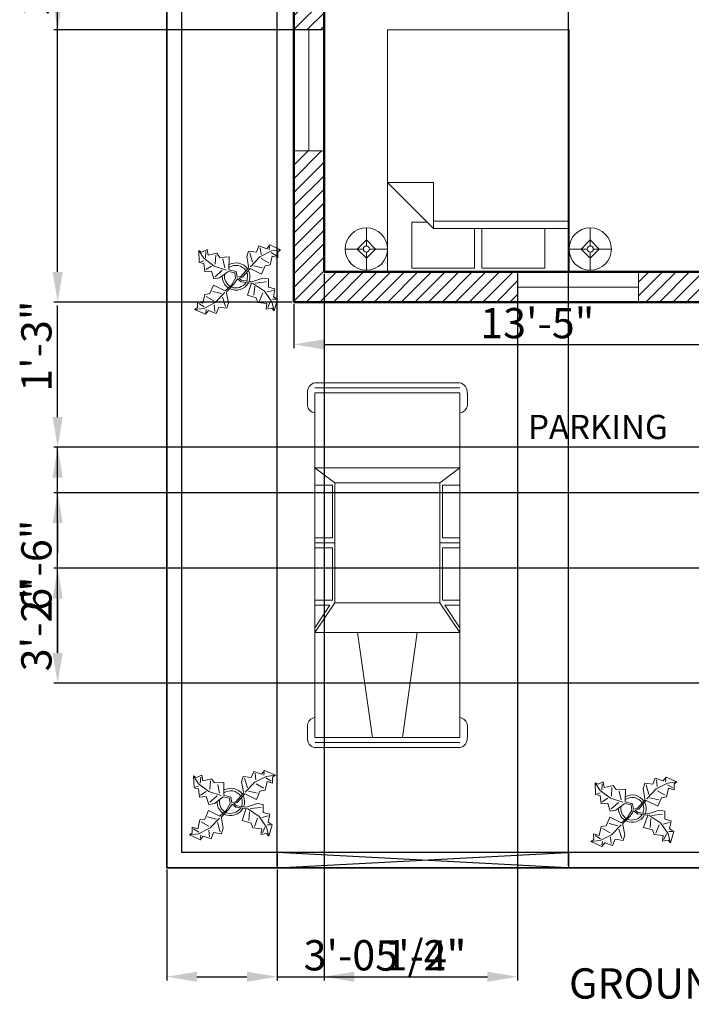
# Model space of a CAD drawing. Units: inches. Extents: x 2206 to 2843, y 1750 to 2489.
# Tile 1 of 8: x 2206 to 2428, y 1750 to 2075. Entities that reach past the tile are written whole.
import ezdxf

# ---------------------------------------------------------------- set-up
doc = ezdxf.new("R2010")
doc.units = ezdxf.units.IN
for name, color, linetype, lineweight in [('A-ANNO-DIMS', 2, 'Continuous', 18), ('A-ANNO-TEXT', 7, 'Continuous', 25), ('A-AREA-IDEN', 7, 'Continuous', 18), ('A-FURN', 21, 'Continuous', 18), ('A-GLAZ', 4, 'Continuous', 18), ('A-WALL', 7, 'Continuous', 50), ('A-WALL-PATT', 252, 'Continuous', 13), ('C-PROP', 7, 'Continuous', 35), ('C-SITE-PKNG', 8, 'Continuous', 18), ('L-PLNT', 92, 'Continuous', 18), ('L-SITE-WALL', 8, 'Continuous', 25)]:
    doc.layers.add(name, color=color, linetype=linetype, lineweight=lineweight)
doc.styles.get("Standard").update_dxf_attribs({"font": 'arial.ttf'})
doc.dimstyles.new('ISO-25', dxfattribs={"dimtxt": 10, "dimasz": 10, "dimexe": 1.25, "dimexo": 0.625, "dimtad": 1, "dimdec": 1, "dimlunit": 3, "dimtxsty": 'Standard', "dimcen": 2.5, "dimadec": 0, "dimazin": 0, "dimtfac": 1, "dimtdec": 1, "dimtmove": 0, "dimatfit": 3, "dimfxl": 1, "dimarcsym": 0})

# ---------------------------------------------------------------- blocks, each defined once
blk = doc.blocks.new('*U2')
for p, q in [((138, 1075), (308, 1075)), ((4818, 1075), (4649, 1075)), ((3, -10), (3, 974)), ((70, -10), (70, 973)), ((138, 973), (410, 973)), ((138, -10), (138, 971)), ((410, 973), (4581, 973)), ((1563, -10), (1563, 973)), ((1563, 973), (1969, 702)), ((1630, 973), (1936, 769)), ((1936, 769), (1936, 973)), ((2003, 973), (2003, 736)), ((2716, 736), (2716, 973)), ((2783, 702), (2783, 973)), ((2851, 973), (2851, 736)), ((3563, 736), (3563, 973)), ((3597, 702), (3801, 973)), ((3801, -10), (3801, 973)), ((4818, 973), (4547, 973)), ((4818, -10), (4818, 971)), ((4886, -10), (4886, 973)), ((4954, -10), (4954, 974)), ((1969, 702), (3597, 702)), ((1969, -10), (1969, 702)), ((2003, 736), (2716, 736)), ((2851, 736), (3563, 736)), ((3597, -10), (3597, 702)), ((138, 193), (1563, 396)), ((3, -11), (3, -995)), ((70, -10), (70, -994)), ((138, -11), (138, -992)), ((1563, -10), (1563, -994)), ((1969, -10), (1969, -723)), ((3597, -10), (3597, -723)), ((3801, -10), (3801, -994)), ((4818, -11), (4818, -992)), ((4886, -10), (4886, -994)), ((4954, -11), (4954, -995)), ((138, -214), (1563, -417)), ((1563, -994), (1969, -723)), ((1630, -994), (1936, -790)), ((1936, -790), (1936, -994)), ((1969, -723), (3597, -723)), ((2003, -994), (2003, -757)), ((2003, -757), (2716, -757)), ((2716, -757), (2716, -994)), ((2783, -723), (2783, -994)), ((2851, -757), (3563, -757)), ((2851, -994), (2851, -757)), ((3563, -757), (3563, -994)), ((3597, -723), (3801, -994)), ((138, -994), (410, -994)), ((410, -994), (4581, -994)), ((4818, -994), (4547, -994)), ((138, -1096), (308, -1096)), ((4818, -1096), (4649, -1096))]:
    blk.add_line(p, q)
for centre, radius, start, end in [((128, 946), 129, 85.6455, 168.0943), ((291, 956), 120, 8.1301, 81.87), ((4665, 956), 120, 98.13, 171.8699), ((4828, 946), 129, 11.9057, 94.3545), ((128, -967), 129, 191.9057, 274.3545), ((291, -977), 120, 278.13, 351.8699), ((4665, -977), 120, 188.1301, 261.87), ((4828, -967), 129, 265.6455, 348.0943)]:
    blk.add_arc(centre, radius, start, end)
blk = doc.blocks.new('Bed - Queen')
for p, q in [((0, -80.00003), (0, 0)), ((0, 0), (59.99999, 0)), ((59.99999, 0), (59.99999, -80.00003)), ((7.99999, -1.2), (28.79998, -1.2)), ((7.99999, -14.4), (7.99999, -1.2)), ((28.79998, -1.2), (28.79998, -14.4)), ((31.19999, -1.2), (51.99999, -1.2)), ((31.19999, -14.4), (31.19999, -1.2)), ((51.99999, -1.2), (51.99999, -16.4)), ((0, -14.4), (44.8, -14.4)), ((59.99999, -29.6), (44.8, -14.4)), ((44.8, -14.4), (44.8, -29.6)), ((44.8, -16.8), (0, -16.8)), ((51.99999, -16.4), (46.79936, -16.4)), ((44.8, -29.6), (59.99999, -29.6)), ((59.99999, -80.00003), (0, -80.00003))]:
    blk.add_line(p, q)
blk = doc.blocks.new('Lamp - Table')
for p, q in [((0, 7), (0, 1)), ((-1, 0), (-7, 0)), ((0, 3), (-3, 0)), ((-3, 0), (0, -3)), ((3, 0), (0, 3)), ((0, -3), (3, 0)), ((1, 0), (7, 0)), ((0, -1), (0, -7))]:
    blk.add_line(p, q)
for radius in [7, 1]:
    blk.add_circle((0, 0), radius)
blk = doc.blocks.new('Plant - Rubber or Philodendron')
for p, q in [((8.8871, 10.7908), (9.9809, 13.4933)), ((9.9809, 13.4933), (13.3837, 12.301)), ((13.3837, 12.301), (14.68, 13.9039)), ((14.5816, 13.2037), (14.3848, 11.8033)), ((14.68, 13.9039), (19.3848, 11.8146)), ((-16.2005, 11.4774), (-13.9899, 8.1064)), ((-16.2005, 11.4774), (-14.8639, 10.7964)), ((-16.0159, 6.3329), (-16.2005, 11.4774)), ((-14.8639, 10.7964), (-12.6195, 11.8975)), ((-13.3174, 8.325), (-13.0735, 11.0065)), ((-12.6195, 11.8975), (-12.1909, 9.4345)), ((-12.1909, 9.4345), (-8.3829, 10.3)), ((-8.8369, 9.409), (-9.0894, 5.6095)), ((-8.3829, 10.3), (-7.0549, 8.501)), ((-7.0549, 8.501), (-3.0284, 8.6941)), ((-3.0284, 8.6941), (-3.0709, 3.1041)), ((4.6914, 8.8812), (5.3859, 11.2828)), ((4.6914, 8.8812), (5.5014, 4.4831)), ((5.3859, 11.2828), (8.8871, 10.7908)), ((5.9878, 10.4842), (7.1971, 6.3869)), ((10.3916, 8.7942), (6.2847, 4.4028)), ((15.3859, 11.3055), (10.3916, 8.7942)), ((10.5828, 12.6946), (10.8893, 9.7953)), ((15.7909, 9.1065), (14.8995, 5.3044)), ((15.2875, 10.6053), (17.5907, 9.2105)), ((19.3848, 11.8146), (15.3859, 11.3055)), ((18.1925, 8.4119), (15.7909, 9.1065)), ((19.3848, 11.8146), (18.1868, 10.9119)), ((18.1868, 10.9119), (18.1925, 8.4119)), ((-14.0069, 5.8704), (-16.0159, 6.3329)), ((-15.3434, 6.5514), (-13.9984, 6.9884)), ((-13.5868, 2.2894), (-14.0069, 5.8704)), ((-13.9899, 8.1064), (-9.5434, 4.7185)), ((-13.1329, 3.1804), (-10.6614, 4.727)), ((-9.5434, 4.7185), (-4.1917, 2.9888)), ((-4.8529, 4.012), (-5.7184, 7.82)), ((5.4346, 3.9146), (5.5014, 4.4831)), ((7.7005, 4.8881), (11.5025, 3.9967)), ((14.2977, 6.1031), (10.9934, 7.9956)), ((12.7005, 4.8994), (11.1089, 1.1958)), ((14.8995, 5.3044), (12.7005, 4.8994)), ((-10.6784, 2.491), (-13.5868, 2.2894)), ((-9.5858, -0.8715), (-10.6784, 2.491)), ((-9.1318, 0.0195), (-5.9793, 2.9025)), ((-7.1228, -0.443), (-3.5248, 2.2131)), ((-3.5248, 2.2131), (-3.3011, 2.4355)), ((-3.3011, 2.4355), (-0.5306, 1.7947)), ((-3.0709, 3.1041), (0.0797, 2.3163)), ((-0.5306, 1.7947), (-0.2255, -0.5527)), ((-0.5306, 1.7947), (-0.5306, 1.7947)), ((0.0797, 2.3163), (0.4866, -0.031)), ((0.4866, -0.031), (2.1141, 0.2298)), ((2.1141, 0.2298), (5.4346, 3.9146)), ((6.1032, 3.6844), (2.8262, -0.031)), ((11.1089, 1.1958), (6.1032, 3.6844)), ((-11.3237, -7.2629), (-9.7321, -3.5593)), ((-9.7321, -3.5593), (-4.7264, -6.0479)), ((-7.1228, -0.443), (-9.5858, -0.8715)), ((-2.019, -3.6148), (-4.7264, -6.0479)), ((-4.0579, -6.2781), (-0.9375, -3.1608)), ((-2.019, -3.6148), (-0.2255, -0.5527)), ((-0.9375, -3.1608), (0.5883, -0.8135)), ((0.5883, -0.8135), (2.2447, -2.0916)), ((2.8262, -0.031), (1.3003, -0.5527)), ((1.3003, -0.5527), (2.4193, -1.4655)), ((2.2447, -2.0916), (6.7108, -2.6626)), ((2.4193, -1.4655), (6.895, -2.1175)), ((4.943, -7.9659), (6.7108, -2.6626)), ((11.6605, -0.5413), (6.895, -2.1175)), ((12.3677, -6.1981), (7.219, -2.6772)), ((8.125, -4.0768), (7.7715, -7.9659)), ((8.3544, -2.7453), (13.1973, -2.1704)), ((11.6605, -0.5413), (14.1354, -0.8948)), ((14.1354, -0.8948), (14.1354, -4.4304)), ((-14.4141, -11.4699), (-13.5228, -7.6679)), ((-13.5228, -7.6679), (-11.3237, -7.2629)), ((-12.921, -8.4665), (-9.6166, -10.359)), ((-6.3237, -7.2516), (-10.1257, -6.3602)), ((-9.0148, -11.1577), (-4.9047, -6.8122)), ((-4.1246, -6.8466), (-4.0579, -6.2781)), ((-3.3146, -11.2447), (-4.1246, -6.8466)), ((8.8321, -9.0266), (4.943, -7.9659)), ((10.2463, -10.4408), (11.6605, -6.9053)), ((15.5496, -10.7943), (12.3677, -6.1981)), ((16.2567, -5.8446), (13.4283, -6.5517)), ((14.1354, -4.4304), (16.9638, -5.1375)), ((16.9638, -5.1375), (16.2567, -8.673)), ((-16.8157, -10.7754), (-14.4141, -11.4699)), ((-16.8101, -13.2754), (-16.8157, -10.7754)), ((-13.9107, -12.9688), (-16.2139, -11.574)), ((-14.0091, -13.669), (-9.0148, -11.1577)), ((-9.206, -15.0581), (-9.5126, -12.1588)), ((-4.611, -12.8477), (-5.8203, -8.7504)), ((-3.3146, -11.2447), (-4.0092, -13.6463)), ((9.5392, -11.1479), (8.8321, -9.0266)), ((13.4283, -11.5015), (9.5392, -11.1479)), ((13.0748, -13.9763), (13.4283, -11.5015)), ((14.8425, -10.7943), (13.7819, -13.2692)), ((16.6103, -14.6834), (15.5496, -10.7943)), ((17.3174, -9.7337), (15.9032, -9.7337)), ((16.2567, -8.673), (18.0245, -9.7337)), ((18.0245, -9.7337), (16.6103, -14.6834)), ((-18.008, -14.1781), (-16.8101, -13.2754)), ((-18.008, -14.1781), (-14.0091, -13.669)), ((-13.3032, -16.2674), (-18.008, -14.1781)), ((-12.0069, -14.6645), (-13.3032, -16.2674)), ((-13.2048, -15.5672), (-13.008, -14.1668)), ((-8.6042, -15.8568), (-12.0069, -14.6645)), ((-7.5103, -13.1543), (-8.6042, -15.8568)), ((-4.0092, -13.6463), (-7.5103, -13.1543)), ((15.5496, -13.6228), (13.0748, -13.9763)), ((16.6103, -14.6834), (15.5496, -13.6228))]:
    blk.add_line(p, q)
for centre, radius, start, end in [((0, 0), 6.1275, 34.37569, 120.1028), ((-0.0601, -0.2075), 5.2461, 33.82192, 124.9414), ((0.0308, 0.1664), 6, 178.6147, 235.1169), ((0.0308, 0.1664), 5, 168.1647, 238.6725), ((-0.2664, 0.1682), 5.2775, 338.4094, 20.03007), ((-0.098, 0.1364), 6.1288, 341.2017, 26.09184), ((-0.0234, 0.3825), 6.1492, 242.5812, 331.2714), ((-0.1102, 0.4886), 5.2883, 247.3711, 327.472)]:
    blk.add_arc(centre, radius, start, end)
blk = doc.blocks.new('*D17')
at = {"layer": 'A-ANNO-DIMS', "color": 0, "lineweight": -2, "transparency": 16777216}
for p, q in [((2296.58, 1981.27), (2296.58, 1966.68)), ((2457.58, 1981.27), (2457.58, 1966.68)), ((2306.58, 1967.93), (2447.58, 1967.93))]:
    blk.add_line(p, q, dxfattribs=at)
at = {"layer": 'A-ANNO-DIMS', "color": 0, "transparency": 16777216}
for points in [[(2306.58, 1969.6), (2306.58, 1966.26), (2296.58, 1967.93)], [(2447.58, 1969.6), (2447.58, 1966.26), (2457.58, 1967.93)]]:
    blk.add_solid(points, dxfattribs=at)
at = {"layer": 'Defpoints', "color": 0, "transparency": 16777216}
for p in [(2296.58, 1981.9), (2457.58, 1981.9), (2457.58, 1967.93)]:
    blk.add_point(p, dxfattribs=at)
at = {"layer": 'A-ANNO-DIMS', "color": 0, "transparency": 16777216, "insert": (2377.08, 1973.66), "char_height": 10, "attachment_point": 5}
blk.add_mtext('13\'-5"', dxfattribs=at)
blk = doc.blocks.new('WIN-40IN')
for p, q in [((10, 40), (0, 40)), ((5, 40), (5, 0)), ((10, 0), (0, 0))]:
    blk.add_line(p, q)
blk = doc.blocks.new('*D58')
at = {"layer": 'A-ANNO-DIMS', "color": 0, "lineweight": -2, "transparency": 16777216}
for p, q in [((2295.95, 2394.9), (2217.28, 2394.9)), ((2218.53, 1991.9), (2218.53, 2384.9)), ((2295.95, 1981.9), (2217.28, 1981.9))]:
    blk.add_line(p, q, dxfattribs=at)
at = {"layer": 'A-ANNO-DIMS', "color": 0, "transparency": 16777216}
for points in [[(2216.86, 2384.9), (2220.2, 2384.9), (2218.53, 2394.9)], [(2216.86, 1991.9), (2220.2, 1991.9), (2218.53, 1981.9)]]:
    blk.add_solid(points, dxfattribs=at)
at = {"layer": 'Defpoints', "color": 0, "transparency": 16777216}
for p in [(2218.53, 2394.9), (2296.58, 2394.9), (2296.58, 1981.9)]:
    blk.add_point(p, dxfattribs=at)
at = {"layer": 'A-ANNO-DIMS', "color": 0, "transparency": 16777216, "insert": (2212.8, 2188.4), "char_height": 10, "attachment_point": 5, "rotation": 90}
blk.add_mtext('34\'-5"', dxfattribs=at)
blk = doc.blocks.new('*D60')
at = {"layer": 'A-ANNO-DIMS', "color": 0, "lineweight": -2, "transparency": 16777216}
for p, q in [((2520.95, 1933.9), (2217.28, 1933.9)), ((2218.53, 1865.9), (2218.53, 1923.9)), ((2520.95, 1855.9), (2217.28, 1855.9))]:
    blk.add_line(p, q, dxfattribs=at)
at = {"layer": 'A-ANNO-DIMS', "color": 0, "transparency": 16777216}
for points in [[(2216.86, 1923.9), (2220.2, 1923.9), (2218.53, 1933.9)], [(2216.86, 1865.9), (2220.2, 1865.9), (2218.53, 1855.9)]]:
    blk.add_solid(points, dxfattribs=at)
at = {"layer": 'Defpoints', "color": 0, "transparency": 16777216}
for p in [(2218.53, 1933.9), (2521.58, 1933.9), (2521.58, 1855.9)]:
    blk.add_point(p, dxfattribs=at)
at = {"layer": 'A-ANNO-DIMS', "color": 0, "transparency": 16777216, "insert": (2212.8, 1894.9), "char_height": 10, "attachment_point": 5, "rotation": 90}
blk.add_mtext('6\'-6"', dxfattribs=at)
blk = doc.blocks.new('*D67')
at = {"layer": 'A-ANNO-DIMS', "color": 0, "lineweight": -2, "transparency": 16777216}
for p, q in [((2305.95, 2111.9), (2217.28, 2111.9)), ((2218.53, 2081.9), (2218.53, 2101.9)), ((2305.95, 2071.9), (2217.28, 2071.9))]:
    blk.add_line(p, q, dxfattribs=at)
at = {"layer": 'A-ANNO-DIMS', "color": 0, "transparency": 16777216}
for points in [[(2216.86, 2101.9), (2220.2, 2101.9), (2218.53, 2111.9)], [(2216.86, 2081.9), (2220.2, 2081.9), (2218.53, 2071.9)]]:
    blk.add_solid(points, dxfattribs=at)
at = {"layer": 'Defpoints', "color": 0, "transparency": 16777216}
for p in [(2218.53, 2111.9), (2306.58, 2111.9), (2306.58, 2071.9)]:
    blk.add_point(p, dxfattribs=at)
at = {"layer": 'A-ANNO-DIMS', "color": 0, "transparency": 16777216, "insert": (2212.8, 2091.9), "char_height": 10, "attachment_point": 5, "rotation": 90}
blk.add_mtext('3\'-4"', dxfattribs=at)
blk = doc.blocks.new('*D68')
at = {"layer": 'A-ANNO-DIMS', "color": 0, "lineweight": -2, "transparency": 16777216}
for p, q in [((2306.58, 1991.27), (2306.58, 1757.6)), ((2370.58, 1991.27), (2370.58, 1757.6)), ((2316.58, 1758.85), (2360.58, 1758.85))]:
    blk.add_line(p, q, dxfattribs=at)
at = {"layer": 'A-ANNO-DIMS', "color": 0, "transparency": 16777216}
for points in [[(2316.58, 1760.52), (2316.58, 1757.18), (2306.58, 1758.85)], [(2360.58, 1760.52), (2360.58, 1757.18), (2370.58, 1758.85)]]:
    blk.add_solid(points, dxfattribs=at)
at = {"layer": 'Defpoints', "color": 0, "transparency": 16777216}
for p in [(2306.58, 1991.9), (2370.58, 1991.9), (2370.58, 1758.85)]:
    blk.add_point(p, dxfattribs=at)
at = {"layer": 'A-ANNO-DIMS', "color": 0, "transparency": 16777216, "insert": (2338.58, 1764.56), "char_height": 10, "attachment_point": 5}
blk.add_mtext('5\'-4"', dxfattribs=at)
blk = doc.blocks.new('*D71')
at = {"layer": 'A-ANNO-DIMS', "color": 0, "lineweight": -2, "transparency": 16777216}
for p, q in [((2218.53, 1943.9), (2218.53, 1980.79)), ((2646.95, 1933.9), (2217.28, 1933.9)), ((2218.53, 1918.9), (2218.53, 1933.9)), ((2656.95, 1918.9), (2217.28, 1918.9)), ((2218.53, 1908.9), (2218.53, 1898.9))]:
    blk.add_line(p, q, dxfattribs=at)
at = {"layer": 'A-ANNO-DIMS', "color": 0, "transparency": 16777216}
for points in [[(2216.86, 1943.9), (2220.2, 1943.9), (2218.53, 1933.9)], [(2216.86, 1908.9), (2220.2, 1908.9), (2218.53, 1918.9)]]:
    blk.add_solid(points, dxfattribs=at)
at = {"layer": 'Defpoints', "color": 0, "transparency": 16777216}
for p in [(2218.53, 1933.9), (2647.58, 1933.9), (2657.58, 1918.9)]:
    blk.add_point(p, dxfattribs=at)
at = {"layer": 'A-ANNO-DIMS', "color": 0, "transparency": 16777216, "insert": (2212.8, 1967.34), "char_height": 10, "attachment_point": 5, "rotation": 90}
blk.add_mtext('1\'-3"', dxfattribs=at)
blk = doc.blocks.new('*D72')
at = {"layer": 'A-ANNO-DIMS', "color": 0, "lineweight": -2, "transparency": 16777216}
for p, q in [((2291.11, 1795.52), (2291.11, 2432.2)), ((2387.37, 1795.52), (2387.37, 2432.2)), ((2301.11, 2430.95), (2377.37, 2430.95))]:
    blk.add_line(p, q, dxfattribs=at)
at = {"layer": 'A-ANNO-DIMS', "color": 0, "transparency": 16777216}
for points in [[(2301.11, 2432.62), (2301.11, 2429.28), (2291.11, 2430.95)], [(2377.37, 2432.62), (2377.37, 2429.28), (2387.37, 2430.95)]]:
    blk.add_solid(points, dxfattribs=at)
at = {"layer": 'Defpoints', "color": 0, "transparency": 16777216}
for p in [(2387.37, 2430.95), (2291.11, 1794.9), (2387.37, 1794.9)]:
    blk.add_point(p, dxfattribs=at)
at = {"layer": 'A-ANNO-DIMS', "color": 0, "transparency": 16777216, "insert": (2339.24, 2436.74), "char_height": 10, "attachment_point": 5}
blk.add_mtext('8\'-0 1/2"', dxfattribs=at)
blk = doc.blocks.new('*D73')
at = {"layer": 'A-ANNO-DIMS', "color": 0, "lineweight": -2, "transparency": 16777216}
for p, q in [((2254.58, 1794.27), (2254.58, 1757.6)), ((2291.11, 1794.27), (2291.11, 1757.6)), ((2264.58, 1758.85), (2281.11, 1758.85)), ((2291.11, 1758.85), (2352.24, 1758.85))]:
    blk.add_line(p, q, dxfattribs=at)
at = {"layer": 'A-ANNO-DIMS', "color": 0, "transparency": 16777216}
for points in [[(2264.58, 1760.52), (2264.58, 1757.18), (2254.58, 1758.85)], [(2281.11, 1760.52), (2281.11, 1757.18), (2291.11, 1758.85)]]:
    blk.add_solid(points, dxfattribs=at)
at = {"layer": 'Defpoints', "color": 0, "transparency": 16777216}
for p in [(2254.58, 1794.9), (2291.11, 1794.9), (2291.11, 1758.85)]:
    blk.add_point(p, dxfattribs=at)
at = {"layer": 'A-ANNO-DIMS', "color": 0, "transparency": 16777216, "insert": (2326.67, 1764.65), "char_height": 10, "attachment_point": 5}
blk.add_mtext('3\'-0 1/2"', dxfattribs=at)
blk = doc.blocks.new('*D75')
at = {"layer": 'A-ANNO-DIMS', "color": 0, "lineweight": -2, "transparency": 16777216}
for p, q in [((2520.95, 1893.9), (2217.28, 1893.9)), ((2218.53, 1883.9), (2218.53, 1865.9)), ((2520.95, 1855.9), (2217.28, 1855.9))]:
    blk.add_line(p, q, dxfattribs=at)
at = {"layer": 'A-ANNO-DIMS', "color": 0, "transparency": 16777216}
for points in [[(2216.86, 1883.9), (2220.2, 1883.9), (2218.53, 1893.9)], [(2216.86, 1865.9), (2220.2, 1865.9), (2218.53, 1855.9)]]:
    blk.add_solid(points, dxfattribs=at)
at = {"layer": 'Defpoints', "color": 0, "transparency": 16777216}
for p in [(2521.58, 1893.9), (2218.53, 1855.9), (2521.58, 1855.9)]:
    blk.add_point(p, dxfattribs=at)
at = {"layer": 'A-ANNO-DIMS', "color": 0, "transparency": 16777216, "insert": (2212.8, 1874.9), "char_height": 10, "attachment_point": 5, "rotation": 90}
blk.add_mtext('3\'-2"', dxfattribs=at)

msp = doc.modelspace()

# ---------------------------------------------------------------- hatches: boundary and pattern name
at = {"layer": 'A-WALL-PATT'}
h = msp.add_hatch(dxfattribs=at)
h.set_pattern_fill('ANSI31', color=256)
h.paths.add_polyline_path([(2710.58, 2394.9), (2296.58, 2394.9), (2296.58, 2335.9), (2306.58, 2335.9), (2306.58, 2384.9), (2479.58, 2384.9), (2652.58, 2384.9), (2700.58, 2384.9), (2700.58, 2300.9), (2690.58, 2300.9), (2690.58, 2290.9), (2710.58, 2290.9)])
h.paths.add_polyline_path([(2306.58, 2295.9), (2296.58, 2295.9), (2296.58, 2225.9), (2306.58, 2225.9), (2306.58, 2241.9)])
h.paths.add_polyline_path([(2306.58, 2111.9), (2306.58, 2132.9), (2296.58, 2132.9), (2296.58, 2071.9), (2306.58, 2071.9)])
h.paths.add_polyline_path([(2306.58, 2197.9), (2296.58, 2197.9), (2296.58, 2160.9), (2306.58, 2160.9), (2306.58, 2176.9)])
h.paths.add_polyline_path([(2370.58, 1991.9), (2306.58, 1991.9), (2306.58, 2031.9), (2296.58, 2031.9), (2296.58, 1981.9), (2370.58, 1981.9)])
h.paths.add_polyline_path([(2479.58, 2066.9), (2474.58, 2066.9), (2474.58, 1991.9), (2410.58, 1991.9), (2410.58, 1981.9), (2479.58, 1981.9)])
h.paths.add_polyline_path([(2539.58, 1943.9), (2479.58, 1943.9), (2479.58, 1944.9), (2469.58, 1944.9), (2469.58, 1933.9), (2539.58, 1933.9)])
h.paths.add_polyline_path([(2657.58, 1997.9), (2647.58, 1997.9), (2647.58, 1943.9), (2647.58, 1918.9), (2657.58, 1918.9)])
h.paths.add_polyline_path([(2647.58, 1943.9), (2587.58, 1943.9), (2587.58, 1933.9), (2647.58, 1933.9)])
h.paths.add_polyline_path([(2657.58, 2158.4), (2647.58, 2158.4), (2647.58, 2104.9), (2647.58, 2045.9), (2657.58, 2045.9)])
h.paths.add_polyline_path([(2657.58, 2204.89), (2647.58, 2204.89), (2647.58, 2188.4), (2657.58, 2188.4)])
h.paths.add_polyline_path([(2657.58, 2246.9), (2647.58, 2246.9), (2647.58, 2234.9), (2657.58, 2234.9)])
h.paths.add_polyline_path([(2662.58, 2300.9), (2652.58, 2300.9), (2652.58, 2346.22), (2647.58, 2346.22), (2647.58, 2290.9), (2662.58, 2290.9)])
h.paths.add_polyline_path([(2647.58, 2246.9), (2524.58, 2246.9), (2524.58, 2241.9), (2647.58, 2241.9)])
h.paths.add_polyline_path([(2351.58, 2246.9), (2306.58, 2246.9), (2306.58, 2241.9), (2351.58, 2241.9)])
h.paths.add_polyline_path([(2429.58, 2246.9), (2381.58, 2246.9), (2381.58, 2241.9), (2390.58, 2241.9), (2390.58, 2181.9), (2306.58, 2181.9), (2306.58, 2176.9), (2390.58, 2176.9), (2390.58, 2116.9), (2381.58, 2116.9), (2381.58, 2111.9), (2474.58, 2111.9), (2474.58, 2102.9), (2479.58, 2102.9), (2479.58, 2104.9), (2479.58, 2116.9), (2395.58, 2116.9), (2395.58, 2176.9), (2395.58, 2241.9), (2429.58, 2241.9)])
h.paths.add_polyline_path([(2479.58, 2384.9), (2474.58, 2384.9), (2474.58, 2246.9), (2465.58, 2246.9), (2465.58, 2241.9), (2479.58, 2241.9), (2488.58, 2241.9), (2488.58, 2246.9), (2479.58, 2246.9)])
h.paths.add_polyline_path([(2657.58, 1870.9), (2647.58, 1870.9), (2647.58, 1855.9), (2511.58, 1855.9), (2511.58, 1845.9), (2657.58, 1845.9)])

# ---------------------------------------------------------------- linework, layer by layer
at = {"layer": 'A-WALL'}
for p, q in [((2296.58, 1981.9), (2296.58, 2394.9)), ((2306.58, 1991.9), (2306.58, 2111.9)), ((2306.58, 1991.9), (2474.58, 1991.9)), ((2296.58, 1981.9), (2479.58, 1981.9))]:
    msp.add_line(p, q, dxfattribs=at)
at = {"layer": 'C-PROP'}
for p, q in [((2254.58, 1794.9), (2254.58, 2394.9)), ((2710.58, 1794.9), (2254.58, 1794.9))]:
    msp.add_line(p, q, dxfattribs=at)
at = {"layer": 'L-SITE-WALL'}
for p, q in [((2259.58, 1799.9), (2259.58, 2384.9)), ((2705.58, 1799.9), (2259.58, 1799.9)), ((2291.11, 1799.9), (2291.11, 1794.9)), ((2291.11, 1794.9), (2387.11, 1799.9)), ((2387.11, 1794.9), (2291.11, 1799.9)), ((2387.37, 1799.9), (2387.37, 1794.9))]:
    msp.add_line(p, q, dxfattribs=at)

# ---------------------------------------------------------------- block references
at = {"layer": 'A-FURN', "rotation": 180}
for name, p in [('Bed - Queen', (2387.58, 1991.9)), ('Lamp - Table', (2394.58, 1999.45))]:
    msp.add_blockref(name, p, dxfattribs=at)
at = {"layer": 'A-FURN', "xscale": -1, "rotation": 180}
msp.add_blockref('Lamp - Table', (2320.58, 1999.45), dxfattribs=at)
at = {"layer": 'A-GLAZ'}
for p, rotation in [((2306.58, 2071.9), 180), ((2370.58, 1991.9), 269.9999999999994)]:
    msp.add_blockref('WIN-40IN', p, dxfattribs=dict(at, rotation=rotation))
at = {"layer": 'C-SITE-PKNG', "xscale": 0.024359920544342, "yscale": 0.024359920544342, "zscale": 0.024359920544342, "rotation": 90}
msp.add_blockref('*U2', (2327.26, 1834.54), dxfattribs=at)
at = {"layer": 'L-PLNT', "xscale": 0.7595985084536371, "yscale": 0.7595985084536371, "zscale": 0.7595985084536371}
for p in [(2277.49, 1990.23), (2275.77, 1816.51), (2408.49, 1814.3)]:
    msp.add_blockref('Plant - Rubber or Philodendron', p, dxfattribs=at)

# ---------------------------------------------------------------- texts
at = {"layer": 'A-ANNO-TEXT', "insert": (2387.56, 1761.63), "char_height": 10, "attachment_point": 1}
msp.add_mtext_dynamic_manual_height_columns('{\\fArial|b1|i0|c0|p34;GROUND FLOOR PLAN}', width=169.89, gutter_width=12.5, heights=[0], dxfattribs=at)
at = {"layer": 'A-AREA-IDEN', "insert": (2374.05, 1944.62), "char_height": 8, "attachment_point": 1}
msp.add_mtext_dynamic_manual_height_columns('PARKING', width=91.9993, gutter_width=12.5, heights=[0], dxfattribs=at)

# ---------------------------------------------------------------- dimensions: what is measured, and where the dimension line sits
at = {"layer": 'A-ANNO-DIMS'}
for base, p1, p2, override, picture, middle in [((2387.37, 2430.95), (2291.11, 1794.9), (2387.37, 1794.9), {"dimdec": 1, "dimlfac": 1, "dimrnd": 0, "dimzin": 1, "dimdsep": 46, "dimlunit": 4, "dimfrac": 2}, '*D72', (2339.24, 2436.74)), ((2370.58, 1758.85), (2306.58, 1991.9), (2370.58, 1991.9), {"dimdec": 1, "dimlfac": 1, "dimrnd": 0, "dimzin": 1, "dimdsep": 46, "dimlunit": 4, "dimfrac": 2}, '*D68', (2338.58, 1764.56)), ((2457.58, 1967.93), (2296.58, 1981.9), (2457.58, 1981.9), {"dimclrd": 0, "dimclre": 0, "dimclrt": 0}, '*D17', (2377.08, 1973.66)), ((2291.11, 1758.85), (2254.58, 1794.9), (2291.11, 1794.9), {"dimdec": 1, "dimlfac": 1, "dimrnd": 0, "dimzin": 1, "dimdsep": 46, "dimlunit": 4, "dimfrac": 2}, '*D73', (2326.67, 1764.65))]:
    dim = msp.add_linear_dim(base=base, p1=p1, p2=p2, dimstyle='ISO-25', override=override, dxfattribs=at)
    dim.commit()
    dim.dimension.update_dxf_attribs({"geometry": picture, "text_midpoint": middle})
for base, p1, p2, picture, middle in [((2218.53, 2394.9), (2296.58, 1981.9), (2296.58, 2394.9), '*D58', (2212.8, 2188.4)), ((2218.53, 2111.9), (2306.58, 2071.9), (2306.58, 2111.9), '*D67', (2212.8, 2091.9)), ((2218.53, 1933.9), (2657.58, 1918.9), (2647.58, 1933.9), '*D71', (2212.8, 1967.34)), ((2218.53, 1933.9), (2521.58, 1855.9), (2521.58, 1933.9), '*D60', (2212.8, 1894.9)), ((2218.53, 1855.9), (2521.58, 1893.9), (2521.58, 1855.9), '*D75', (2212.8, 1874.9))]:
    dim = msp.add_linear_dim(base=base, p1=p1, p2=p2, angle=90, dimstyle='ISO-25', override={"dimdec": 1, "dimlfac": 1, "dimrnd": 0, "dimzin": 1, "dimdsep": 46, "dimlunit": 4, "dimfrac": 2}, dxfattribs=at)
    dim.commit()
    dim.dimension.update_dxf_attribs({"geometry": picture, "text_midpoint": middle})

doc.saveas('drawing.dxf')
